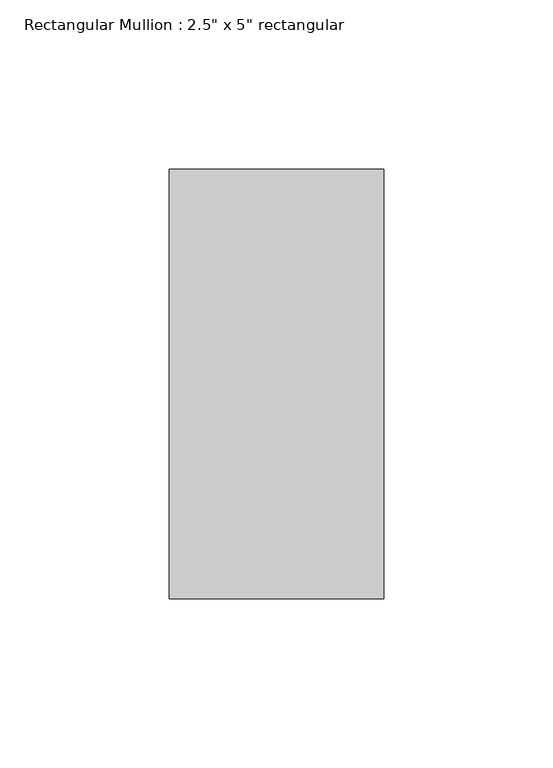
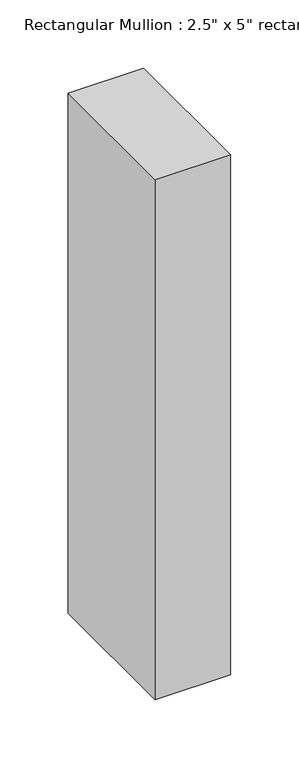
"""IFC4 building model written with IfcOpenShell, lengths in millimetres: member geometry."""

from ifc_helpers import new_model, si_unit, frame, origin, place, context, project, spatial, polyline, outline, extrude, source, transform, mapped, element, save


def member_5535eeb3(model_context):
    return source(origin(), model_context, "Body", "SweptSolid", [
        extrude(outline(polyline([(0.0, 63.5), (0.0, -63.5), (-63.5, -63.5), (-63.5, 63.5), (0.0, 63.5)])), frame((0.0, 0.0, -463.55), z_axis=(0.0, 0.0, 1.0), x_axis=(1.0, 0.0, 0.0)), (0.0, 0.0, 1.0), 463.55),
    ])


if __name__ == "__main__":
    model = new_model("IFC4")
    model_context = context("Model", 3, world=origin())
    ifc_project = project(units=[si_unit("LENGTHUNIT", "METRE", prefix="MILLI")], contexts=[model_context])
    site = spatial("IfcSite", under=ifc_project)
    building = spatial("IfcBuilding", under=site)
    placement = place(None, origin())
    member_shape = member_5535eeb3(model_context)
    element("IfcMember", 1, ObjectType="Rectangular Mullion : 2.5\" x 5\" rectangular", at=placement, inside=building, context=model_context, shape_type="MappedRepresentation", body=[
        mapped(member_shape, transform((0.0, 0.0, 0.0), x_axis=(1.0, 0.0, 0.0), y_axis=(0.0, 1.0, 0.0), z_axis=(0.0, 0.0, 1.0))),
    ])
    save(model, "model.ifc")

# Revit data of these elements
# Type "Rectangular Mullion : 2.5\" x 5\" rectangular"
#   built-in parameter 1007304 = 0.416667 (stored number, unit not read)
#   built-in parameter 1007301 = 0.104167 (stored number, unit not read)
#   built-in parameter 1007300 = 0.104167 (stored number, unit not read)
# Element 1 (IfcMember, "Rectangular Mullion : 2.5\" x 5\" rectangular")
#   Materials on its faces: "Aluminum"
# Materials
#   "Aluminum": class "Metal", colour RGB 247 247 247, transparency 0, Description = "Aluminum 6061", Cost = 0
